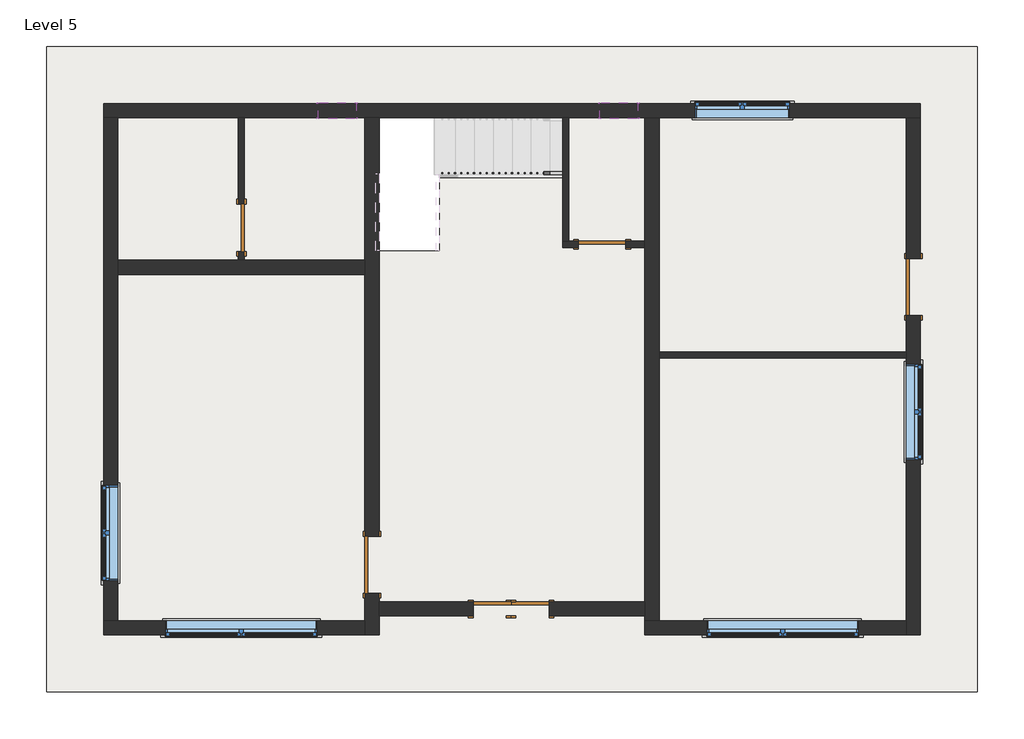
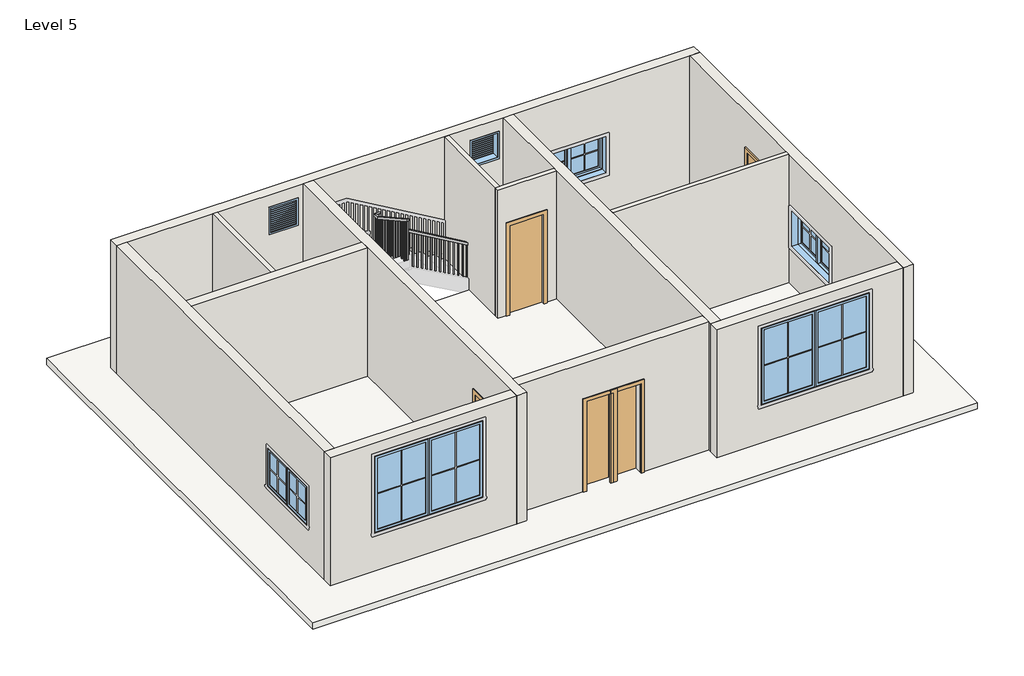
# One storey, part 1 of 2: 13 walls, 7 windows, 6 doors, 1 railing, 1 roof.
"""IFC4 building model written with IfcOpenShell, lengths in millimetres."""

from ifc_helpers import new_model, si_unit, frame, origin, place, context, project, spatial, polyline, outline, extrude, faceted_brep, transform, mapped, element, save
from components import single_flush_door_2_4a3212df, single_flush_door_2_0d3b4037, door_270f2424, door_aa9e95e7, single_flush_door_3_a90ba1ad, window_casement_double_c1d95f0f, window_casement_double_9ae172a2, window_f2d8fef0

model = new_model("IFC4")

# Units and contexts
model_context = context("Model", 3, world=origin())
ifc_project = project(units=[si_unit("LENGTHUNIT", "METRE", prefix="MILLI")], contexts=[model_context])

# Site, building, storey
site = spatial("IfcSite", under=ifc_project)
building = spatial("IfcBuilding", under=site)
storey = spatial("IfcBuildingStorey", under=building, Name="Level 5", Elevation=12649.2)

# Doors
placement = place(None, origin())
single_flush_door_2_shape = single_flush_door_2_4a3212df(model_context)
element("IfcDoor", 1, ObjectType="Single-Flush : DOOR 2'", at=placement, inside=storey, context=model_context, shape_type="MappedRepresentation", body=[
    mapped(single_flush_door_2_shape, transform((-1572.7415084, -2604.3618005, 12649.2), x_axis=(-1.0, 0.0, 0.0), y_axis=(0.0, -1.0, 0.0), z_axis=(0.0, 0.0, 1.0))),
])
single_flush_door_2_2_shape = single_flush_door_2_0d3b4037(model_context)
element("IfcDoor", 2, ObjectType="Single-Flush : DOOR 2'", at=placement, inside=storey, context=model_context, shape_type="MappedRepresentation", body=[
    mapped(single_flush_door_2_2_shape, transform((-963.1415084, -2604.3618005, 12649.2), x_axis=(1.0, 0.0, 0.0), y_axis=(0.0, 1.0, 0.0), z_axis=(0.0, 0.0, 1.0))),
])
door_shape = door_270f2424(model_context)
element("IfcDoor", 3, ObjectType="Single-Flush : DOOR 2'6\"", at=placement, inside=storey, context=model_context, shape_type="MappedRepresentation", body=[
    mapped(door_shape, transform((-5598.6415084, 3517.0381995, 12649.2), x_axis=(0.0, -1.0, 0.0), y_axis=(1.0, 0.0, 0.0), z_axis=(0.0, 0.0, 1.0))),
])
door_2_shape = door_aa9e95e7(model_context)
element("IfcDoor", 4, ObjectType="Single-Flush : DOOR 2'6\"", at=placement, inside=storey, context=model_context, shape_type="MappedRepresentation", body=[
    mapped(door_2_shape, transform((192.5584916, 3250.3381995, 12649.2), x_axis=(-1.0, 0.0, 0.0), y_axis=(0.0, -1.0, 0.0), z_axis=(0.0, 0.0, 1.0))),
])
single_flush_door_3_shape = single_flush_door_3_a90ba1ad(model_context)
element("IfcDoor", 5, ObjectType="Single-Flush : DOOR 3'", at=placement, inside=storey, context=model_context, shape_type="MappedRepresentation", body=[
    mapped(single_flush_door_3_shape, transform((-3503.1415084, -1893.1618005, 12649.2), x_axis=(0.0, -1.0, 0.0), y_axis=(1.0, 0.0, 0.0), z_axis=(0.0, 0.0, 1.0))),
])
element("IfcDoor", 6, ObjectType="Single-Flush : DOOR 3'", at=placement, inside=storey, context=model_context, shape_type="MappedRepresentation", body=[
    mapped(single_flush_door_3_shape, transform((5183.6584916, 2564.5381995, 12649.2), x_axis=(0.0, -1.0, 0.0), y_axis=(1.0, 0.0, 0.0), z_axis=(0.0, 0.0, 1.0))),
])

# Railing
element("IfcRailing", 7, ObjectType="Handrail - Rectangular", at=placement, inside=storey, context=model_context, shape_type="SolidModel", body=[
    faceted_brep([(-442.4415084, 4368.3146777, 13732.9333333), (-442.4415084, 4368.3146777, 13674.1219871), (-442.4415084, 4419.1146777, 13674.1219871), (-442.4415084, 4419.1146777, 13732.9333333), (-2398.2415084, 4368.3146777, 14873.8166667), (-2449.0415084, 4368.3146777, 14844.6386538), (-2449.0415084, 4419.1146777, 14844.6386538), (-2398.2415084, 4419.1146777, 14873.8166667), (-2398.2415084, 4368.3146777, 15129.9202697), (-2449.0415084, 4368.3146777, 15079.1202697), (-2449.0415084, 4419.1146777, 15079.1202697), (-2398.2415084, 4419.1146777, 15129.9202697), (-2474.4415084, 4368.3146777, 15129.9202697), (-2474.4415084, 4368.3146777, 15079.1202697), (-2525.2415084, 4419.1146777, 15079.1202697), (-2525.2415084, 4419.1146777, 15129.9202697), (-2474.4415084, 4292.1146777, 15129.9202697), (-2474.4415084, 4278.9546266, 15079.1202697), (-2525.2415084, 4278.9546266, 15079.1202697), (-2525.2415084, 4292.1146777, 15129.9202697), (-2474.4415084, 3148.7383287, 15764.9333333), (-2525.2415084, 3148.7383287, 15764.9333333), (-2525.2415084, 3148.7383287, 15706.82445), (-2474.4415084, 3148.7383287, 15706.82445)], [[[0, 1, 2, 3]], [[1, 0, 4, 5]], [[2, 1, 5, 6]], [[3, 2, 6, 7]], [[0, 3, 7, 4]], [[5, 4, 8, 9]], [[6, 5, 9, 10]], [[7, 6, 10, 11]], [[4, 7, 11, 8]], [[9, 8, 12, 13]], [[10, 9, 13, 14]], [[11, 10, 14, 15]], [[8, 11, 15, 12]], [[13, 12, 16, 17]], [[14, 13, 17, 18]], [[15, 14, 18, 19]], [[12, 15, 19, 16]], [[20, 21, 22, 23]], [[17, 16, 20, 23]], [[18, 17, 23, 22]], [[19, 18, 22, 21]], [[16, 19, 21, 20]]]),
    extrude(outline(polyline([(3184.0396777, 15687.3754052), (3184.0396777, 14681.2), (3164.9896777, 14681.2), (3164.9896777, 15697.9554726), (3184.0396777, 15687.3754052)])), frame((-2509.3665084, 0.0, 0.0), z_axis=(1.0, 0.0, 0.0), x_axis=(0.0, 1.0, 0.0)), (0.0, 0.0, 1.0), 19.05),
    extrude(outline(polyline([(3285.6396777, 15630.9483789), (3285.6396777, 14681.2), (3266.5896777, 14681.2), (3266.5896777, 15641.5284463), (3285.6396777, 15630.9483789)])), frame((-2509.3665084, 0.0, 0.0), z_axis=(1.0, 0.0, 0.0), x_axis=(0.0, 1.0, 0.0)), (0.0, 0.0, 1.0), 19.05),
    extrude(outline(polyline([(3387.2396777, 15574.5213526), (3387.2396777, 14681.2), (3368.1896777, 14681.2), (3368.1896777, 15585.1014201), (3387.2396777, 15574.5213526)])), frame((-2509.3665084, 0.0, 0.0), z_axis=(1.0, 0.0, 0.0), x_axis=(0.0, 1.0, 0.0)), (0.0, 0.0, 1.0), 19.05),
    extrude(outline(polyline([(3488.8396777, 15518.0420718), (3488.8396777, 14511.8666667), (3469.7896777, 14511.8666667), (3469.7896777, 15528.6221392), (3488.8396777, 15518.0420718)])), frame((-2509.3665084, 0.0, 0.0), z_axis=(1.0, 0.0, 0.0), x_axis=(0.0, 1.0, 0.0)), (0.0, 0.0, 1.0), 19.05),
    extrude(outline(polyline([(3590.4396777, 15461.6150456), (3590.4396777, 14511.8666667), (3571.3896777, 14511.8666667), (3571.3896777, 15472.195113), (3590.4396777, 15461.6150456)])), frame((-2509.3665084, 0.0, 0.0), z_axis=(1.0, 0.0, 0.0), x_axis=(0.0, 1.0, 0.0)), (0.0, 0.0, 1.0), 19.05),
    extrude(outline(polyline([(3692.0396777, 15405.1880193), (3692.0396777, 14511.8666667), (3672.9896777, 14511.8666667), (3672.9896777, 15415.7680867), (3692.0396777, 15405.1880193)])), frame((-2509.3665084, 0.0, 0.0), z_axis=(1.0, 0.0, 0.0), x_axis=(0.0, 1.0, 0.0)), (0.0, 0.0, 1.0), 19.05),
    extrude(outline(polyline([(3793.6396777, 15348.7087385), (3793.6396777, 14342.5333333), (3774.5896777, 14342.5333333), (3774.5896777, 15359.2888059), (3793.6396777, 15348.7087385)])), frame((-2509.3665084, 0.0, 0.0), z_axis=(1.0, 0.0, 0.0), x_axis=(0.0, 1.0, 0.0)), (0.0, 0.0, 1.0), 19.05),
    extrude(outline(polyline([(3895.2396777, 15292.2817122), (3895.2396777, 14342.5333333), (3876.1896777, 14342.5333333), (3876.1896777, 15302.8617797), (3895.2396777, 15292.2817122)])), frame((-2509.3665084, 0.0, 0.0), z_axis=(1.0, 0.0, 0.0), x_axis=(0.0, 1.0, 0.0)), (0.0, 0.0, 1.0), 19.05),
    extrude(outline(polyline([(3996.8396777, 15235.854686), (3996.8396777, 14342.5333333), (3977.7896777, 14342.5333333), (3977.7896777, 15246.4347534), (3996.8396777, 15235.854686)])), frame((-2509.3665084, 0.0, 0.0), z_axis=(1.0, 0.0, 0.0), x_axis=(0.0, 1.0, 0.0)), (0.0, 0.0, 1.0), 19.05),
    extrude(outline(polyline([(4098.4396777, 15179.3754052), (4098.4396777, 14173.2), (4079.3896777, 14173.2), (4079.3896777, 15189.9554726), (4098.4396777, 15179.3754052)])), frame((-2509.3665084, 0.0, 0.0), z_axis=(1.0, 0.0, 0.0), x_axis=(0.0, 1.0, 0.0)), (0.0, 0.0, 1.0), 19.05),
    extrude(outline(polyline([(4200.0396777, 15122.9483789), (4200.0396777, 14173.2), (4180.9896777, 14173.2), (4180.9896777, 15133.5284463), (4200.0396777, 15122.9483789)])), frame((-2509.3665084, 0.0, 0.0), z_axis=(1.0, 0.0, 0.0), x_axis=(0.0, 1.0, 0.0)), (0.0, 0.0, 1.0), 19.05),
    extrude(outline(polyline([(4301.6396777, 15066.5213526), (4301.6396777, 14173.2), (4282.5896777, 14173.2), (4282.5896777, 15077.1014201), (4301.6396777, 15066.5213526)])), frame((-2509.3665084, 0.0, 0.0), z_axis=(1.0, 0.0, 0.0), x_axis=(0.0, 1.0, 0.0)), (0.0, 0.0, 1.0), 19.05),
    extrude(outline(polyline([(-2464.9165084, 4384.1896777), (-2483.9665084, 4384.1896777), (-2483.9665084, 4403.2396777), (-2464.9165084, 4403.2396777), (-2464.9165084, 4384.1896777)])), frame((0.0, 0.0, 14003.8666667), z_axis=(0.0, 0.0, 1.0), x_axis=(1.0, 0.0, 0.0)), (0.0, 0.0, 1.0), 1075.253603),
    extrude(outline(polyline([(14805.7449038, -2382.3665084), (13834.5333333, -2382.3665084), (13834.5333333, -2363.3165084), (14794.6324038, -2363.3165084), (14805.7449038, -2382.3665084)])), frame((0.0, 4384.1896777, 0.0), z_axis=(0.0, 1.0, 0.0), x_axis=(0.0, 0.0, 1.0)), (0.0, 0.0, 1.0), 19.05),
    extrude(outline(polyline([(14746.4782371, -2280.7665084), (13834.5333333, -2280.7665084), (13834.5333333, -2261.7165084), (14735.3657371, -2261.7165084), (14746.4782371, -2280.7665084)])), frame((0.0, 4384.1896777, 0.0), z_axis=(0.0, 1.0, 0.0), x_axis=(0.0, 0.0, 1.0)), (0.0, 0.0, 1.0), 19.05),
    extrude(outline(polyline([(14687.2115704, -2179.1665084), (13834.5333333, -2179.1665084), (13834.5333333, -2160.1165084), (14676.0990704, -2160.1165084), (14687.2115704, -2179.1665084)])), frame((0.0, 4384.1896777, 0.0), z_axis=(0.0, 1.0, 0.0), x_axis=(0.0, 0.0, 1.0)), (0.0, 0.0, 1.0), 19.05),
    extrude(outline(polyline([(14627.9449038, -2077.5665084), (13665.2, -2077.5665084), (13665.2, -2058.5165084), (14616.8324038, -2058.5165084), (14627.9449038, -2077.5665084)])), frame((0.0, 4384.1896777, 0.0), z_axis=(0.0, 1.0, 0.0), x_axis=(0.0, 0.0, 1.0)), (0.0, 0.0, 1.0), 19.05),
    extrude(outline(polyline([(14568.6782371, -1975.9665084), (13665.2, -1975.9665084), (13665.2, -1956.9165084), (14557.5657371, -1956.9165084), (14568.6782371, -1975.9665084)])), frame((0.0, 4384.1896777, 0.0), z_axis=(0.0, 1.0, 0.0), x_axis=(0.0, 0.0, 1.0)), (0.0, 0.0, 1.0), 19.05),
    extrude(outline(polyline([(14509.4115704, -1874.3665084), (13665.2, -1874.3665084), (13665.2, -1855.3165084), (14498.2990704, -1855.3165084), (14509.4115704, -1874.3665084)])), frame((0.0, 4384.1896777, 0.0), z_axis=(0.0, 1.0, 0.0), x_axis=(0.0, 0.0, 1.0)), (0.0, 0.0, 1.0), 19.05),
    extrude(outline(polyline([(14450.1449038, -1772.7665084), (13495.8666667, -1772.7665084), (13495.8666667, -1753.7165084), (14439.0324038, -1753.7165084), (14450.1449038, -1772.7665084)])), frame((0.0, 4384.1896777, 0.0), z_axis=(0.0, 1.0, 0.0), x_axis=(0.0, 0.0, 1.0)), (0.0, 0.0, 1.0), 19.05),
    extrude(outline(polyline([(14390.8782371, -1671.1665084), (13495.8666667, -1671.1665084), (13495.8666667, -1652.1165084), (14379.7657371, -1652.1165084), (14390.8782371, -1671.1665084)])), frame((0.0, 4384.1896777, 0.0), z_axis=(0.0, 1.0, 0.0), x_axis=(0.0, 0.0, 1.0)), (0.0, 0.0, 1.0), 19.05),
    extrude(outline(polyline([(14331.6115704, -1569.5665084), (13495.8666667, -1569.5665084), (13495.8666667, -1550.5165084), (14320.4990704, -1550.5165084), (14331.6115704, -1569.5665084)])), frame((0.0, 4384.1896777, 0.0), z_axis=(0.0, 1.0, 0.0), x_axis=(0.0, 0.0, 1.0)), (0.0, 0.0, 1.0), 19.05),
    extrude(outline(polyline([(14272.3449038, -1467.9665084), (13326.5333333, -1467.9665084), (13326.5333333, -1448.9165084), (14261.2324038, -1448.9165084), (14272.3449038, -1467.9665084)])), frame((0.0, 4384.1896777, 0.0), z_axis=(0.0, 1.0, 0.0), x_axis=(0.0, 0.0, 1.0)), (0.0, 0.0, 1.0), 19.05),
    extrude(outline(polyline([(14213.0782371, -1366.3665084), (13326.5333333, -1366.3665084), (13326.5333333, -1347.3165084), (14201.9657371, -1347.3165084), (14213.0782371, -1366.3665084)])), frame((0.0, 4384.1896777, 0.0), z_axis=(0.0, 1.0, 0.0), x_axis=(0.0, 0.0, 1.0)), (0.0, 0.0, 1.0), 19.05),
    extrude(outline(polyline([(14153.8115704, -1264.7665084), (13326.5333333, -1264.7665084), (13326.5333333, -1245.7165084), (14142.6990704, -1245.7165084), (14153.8115704, -1264.7665084)])), frame((0.0, 4384.1896777, 0.0), z_axis=(0.0, 1.0, 0.0), x_axis=(0.0, 0.0, 1.0)), (0.0, 0.0, 1.0), 19.05),
    extrude(outline(polyline([(14094.5449038, -1163.1665084), (13157.2, -1163.1665084), (13157.2, -1144.1165084), (14083.4324038, -1144.1165084), (14094.5449038, -1163.1665084)])), frame((0.0, 4384.1896777, 0.0), z_axis=(0.0, 1.0, 0.0), x_axis=(0.0, 0.0, 1.0)), (0.0, 0.0, 1.0), 19.05),
    extrude(outline(polyline([(14035.2782371, -1061.5665084), (13157.2, -1061.5665084), (13157.2, -1042.5165084), (14024.1657371, -1042.5165084), (14035.2782371, -1061.5665084)])), frame((0.0, 4384.1896777, 0.0), z_axis=(0.0, 1.0, 0.0), x_axis=(0.0, 0.0, 1.0)), (0.0, 0.0, 1.0), 19.05),
    extrude(outline(polyline([(13976.0115704, -959.9665084), (13157.2, -959.9665084), (13157.2, -940.9165084), (13964.8990704, -940.9165084), (13976.0115704, -959.9665084)])), frame((0.0, 4384.1896777, 0.0), z_axis=(0.0, 1.0, 0.0), x_axis=(0.0, 0.0, 1.0)), (0.0, 0.0, 1.0), 19.05),
    extrude(outline(polyline([(13916.7449038, -858.3665084), (12987.8666667, -858.3665084), (12987.8666667, -839.3165084), (13905.6324038, -839.3165084), (13916.7449038, -858.3665084)])), frame((0.0, 4384.1896777, 0.0), z_axis=(0.0, 1.0, 0.0), x_axis=(0.0, 0.0, 1.0)), (0.0, 0.0, 1.0), 19.05),
    extrude(outline(polyline([(13857.4782371, -756.7665084), (12987.8666667, -756.7665084), (12987.8666667, -737.7165084), (13846.3657371, -737.7165084), (13857.4782371, -756.7665084)])), frame((0.0, 4384.1896777, 0.0), z_axis=(0.0, 1.0, 0.0), x_axis=(0.0, 0.0, 1.0)), (0.0, 0.0, 1.0), 19.05),
    extrude(outline(polyline([(13798.2115704, -655.1665084), (12987.8666667, -655.1665084), (12987.8666667, -636.1165084), (13787.0990704, -636.1165084), (13798.2115704, -655.1665084)])), frame((0.0, 4384.1896777, 0.0), z_axis=(0.0, 1.0, 0.0), x_axis=(0.0, 0.0, 1.0)), (0.0, 0.0, 1.0), 19.05),
    extrude(outline(polyline([(13738.9449038, -553.5665084), (12818.5333333, -553.5665084), (12818.5333333, -534.5165084), (13727.8324038, -534.5165084), (13738.9449038, -553.5665084)])), frame((0.0, 4384.1896777, 0.0), z_axis=(0.0, 1.0, 0.0), x_axis=(0.0, 0.0, 1.0)), (0.0, 0.0, 1.0), 19.05),
    extrude(outline(polyline([(-2490.3165084, 4384.1896777), (-2509.3665084, 4384.1896777), (-2509.3665084, 4403.2396777), (-2490.3165084, 4403.2396777), (-2490.3165084, 4384.1896777)])), frame((0.0, 0.0, 14003.8666667), z_axis=(0.0, 0.0, 1.0), x_axis=(1.0, 0.0, 0.0)), (0.0, 0.0, 1.0), 1075.253603),
    extrude(outline(polyline([(3167.7883287, 15696.2443826), (3167.7883287, 14681.2), (3148.7383287, 14681.2), (3148.7383287, 15706.82445), (3167.7883287, 15696.2443826)])), frame((-2509.3665084, 0.0, 0.0), z_axis=(1.0, 0.0, 0.0), x_axis=(0.0, 1.0, 0.0)), (0.0, 0.0, 1.0), 19.05),
    extrude(outline(polyline([(13685.2344871, -461.4915084), (12818.5333333, -461.4915084), (12818.5333333, -442.4415084), (13674.1219871, -442.4415084), (13685.2344871, -461.4915084)])), frame((0.0, 4384.1896777, 0.0), z_axis=(0.0, 1.0, 0.0), x_axis=(0.0, 0.0, 1.0)), (0.0, 0.0, 1.0), 19.05),
])

# Roof
element("IfcRoof", 8, ObjectType="ROOF 6\"", at=placement, inside=storey, context=model_context, shape_type="SweptSolid", body=[
    extrude(outline(polyline([(-8722.8415084, -3937.8618005), (-8722.8415084, 6425.3381995), (6212.3584916, 6425.3381995), (6212.3584916, -3937.8618005), (-8722.8415084, -3937.8618005)]), holes=[polyline([(-3439.6415084, 5333.1381995), (-3439.6415084, 3148.7383287), (-2423.6415084, 3148.7383287), (-2423.6415084, 4317.5146777), (-442.4415084, 4317.5146777), (-442.4415084, 5333.1381995), (-3439.6415084, 5333.1381995)])]), frame((0.0, 0.0, 12496.8), z_axis=(0.0, 0.0, 1.0), x_axis=(1.0, 0.0, 0.0)), (0.0, 0.0, 1.0), 152.4),
])

# Walls
element("IfcWall", 9, ObjectType="WALL 4\"", at=placement, inside=storey, context=model_context, shape_type="SweptSolid", body=[
    extrude(outline(polyline([(3136.0381995, 14782.8), (3136.0381995, 12649.2), (2996.3381995, 12649.2), (2996.3381995, 15697.2), (5282.3381995, 15697.2), (5282.3381995, 12649.2), (3898.0381995, 12649.2), (3898.0381995, 14782.8), (3136.0381995, 14782.8)])), frame((-5649.4415084, 0.0, 0.0), z_axis=(1.0, 0.0, 0.0), x_axis=(0.0, 1.0, 0.0)), (0.0, 0.0, 1.0), 101.6),
])
element("IfcWall", 10, ObjectType="WALL 4\"", at=placement, inside=storey, context=model_context, shape_type="Brep", body=[
    faceted_brep([(-188.4415084, 3301.1381995, 14782.8), (-188.4415084, 3301.1381995, 12649.2), (-340.8415084, 3301.1381995, 12649.2), (-442.4415084, 3301.1381995, 12649.2), (-442.4415084, 3301.1381995, 15697.2), (-340.8415084, 3301.1381995, 15697.2), (878.3584916, 3301.1381995, 15697.2), (878.3584916, 3301.1381995, 12649.2), (573.5584916, 3301.1381995, 12649.2), (573.5584916, 3301.1381995, 14782.8), (-442.4415084, 3199.5381995, 12649.2), (-188.4415084, 3199.5381995, 12649.2), (-188.4415084, 3199.5381995, 14782.8), (573.5584916, 3199.5381995, 14782.8), (573.5584916, 3199.5381995, 12649.2), (878.3584916, 3199.5381995, 12649.2), (878.3584916, 3199.5381995, 15697.2), (-442.4415084, 3199.5381995, 15697.2)], [[[0, 1, 2, 3, 4, 5, 6, 7, 8, 9]], [[10, 11, 12, 13, 14, 15, 16, 17]], [[8, 7, 15, 14]], [[3, 2, 1, 11, 10]], [[7, 6, 16, 15]], [[4, 3, 10, 17]], [[12, 11, 1, 0]], [[13, 12, 0, 9]], [[14, 13, 9, 8]], [[6, 5, 4, 17, 16]]]),
])
element("IfcWall", 11, ObjectType="WALL 4\"", at=placement, inside=storey, context=model_context, shape_type="Brep", body=[
    faceted_brep([(-340.8415084, 3301.1381995, 12649.2), (-340.8415084, 5282.3381995, 12649.2), (-340.8415084, 5282.3381995, 15697.2), (-340.8415084, 3301.1381995, 15697.2), (-442.4415084, 3301.1381995, 12649.2), (-442.4415084, 3301.1381995, 15697.2), (-442.4415084, 4317.5146777, 15697.2), (-442.4415084, 5282.3381995, 15697.2), (-442.4415084, 5282.3381995, 12649.2)], [[[0, 1, 2, 3]], [[4, 5, 6, 7, 8]], [[1, 0, 4, 8]], [[0, 3, 5, 4]], [[2, 1, 8, 7]], [[3, 2, 7, 6, 5]]]),
])
element("IfcWall", 12, ObjectType="WALL 4\"", at=placement, inside=storey, context=model_context, shape_type="SweptSolid", body=[
    extrude(outline(polyline([(1106.9584916, 1523.1381995), (5069.3584916, 1523.1381995), (5069.3584916, 1421.5381995), (1106.9584916, 1421.5381995), (1106.9584916, 1523.1381995)])), frame((0.0, 0.0, 12649.2), z_axis=(0.0, 0.0, 1.0), x_axis=(1.0, 0.0, 0.0)), (0.0, 0.0, 1.0), 3048.0),
])
element("IfcWall", 13, ObjectType="WALL 9\"", at=placement, inside=storey, context=model_context, shape_type="Brep", body=[
    faceted_brep([(-7808.4415084, 5282.3381995, 12649.2), (-7579.8415084, 5282.3381995, 12649.2), (-5649.4415084, 5282.3381995, 12649.2), (-5547.8415084, 5282.3381995, 12649.2), (-3617.4415084, 5282.3381995, 12649.2), (-3388.8415084, 5282.3381995, 12649.2), (-442.4415084, 5282.3381995, 12649.2), (-340.8415084, 5282.3381995, 12649.2), (878.3584916, 5282.3381995, 12649.2), (1106.9584916, 5282.3381995, 12649.2), (5069.3584916, 5282.3381995, 12649.2), (5297.9584916, 5282.3381995, 12649.2), (5297.9584916, 5282.3381995, 15697.2), (5069.3584916, 5282.3381995, 15697.2), (1106.9584916, 5282.3381995, 15697.2), (878.3584916, 5282.3381995, 15697.2), (-340.8415084, 5282.3381995, 15697.2), (-442.4415084, 5282.3381995, 15697.2), (-3388.8415084, 5282.3381995, 15697.2), (-3617.4415084, 5282.3381995, 15697.2), (-5547.8415084, 5282.3381995, 15697.2), (-5649.4415084, 5282.3381995, 15697.2), (-7579.8415084, 5282.3381995, 15697.2), (-7808.4415084, 5282.3381995, 15697.2), (3202.4584916, 5282.3381995, 14478.0), (3202.4584916, 5282.3381995, 13563.6), (1678.4584916, 5282.3381995, 13563.6), (1678.4584916, 5282.3381995, 14478.0), (154.4584916, 5282.3381995, 15392.4), (764.0584916, 5282.3381995, 15392.4), (764.0584916, 5282.3381995, 14782.8), (154.4584916, 5282.3381995, 14782.8), (-3757.1415084, 5282.3381995, 15392.4), (-3757.1415084, 5282.3381995, 14782.8), (-4366.7415084, 5282.3381995, 14782.8), (-4366.7415084, 5282.3381995, 15392.4), (-7808.4415084, 5510.9381995, 12649.2), (-7808.4415084, 5510.9381995, 15697.2), (5297.9584916, 5510.9381995, 15697.2), (5297.9584916, 5510.9381995, 12649.2), (3202.4584916, 5510.9381995, 14478.0), (1678.4584916, 5510.9381995, 14478.0), (1678.4584916, 5510.9381995, 13563.6), (3202.4584916, 5510.9381995, 13563.6), (154.4584916, 5510.9381995, 15392.4), (154.4584916, 5510.9381995, 14782.8), (764.0584916, 5510.9381995, 14782.8), (764.0584916, 5510.9381995, 15392.4), (-3757.1415084, 5510.9381995, 15392.4), (-4366.7415084, 5510.9381995, 15392.4), (-4366.7415084, 5510.9381995, 14782.8), (-3757.1415084, 5510.9381995, 14782.8)], [[[0, 1, 2, 3, 4, 5, 6, 7, 8, 9, 10, 11, 12, 13, 14, 15, 16, 17, 18, 19, 20, 21, 22, 23], [24, 25, 26, 27], [28, 29, 30, 31], [32, 33, 34, 35]], [[36, 37, 38, 39], [40, 41, 42, 43], [44, 45, 46, 47], [48, 49, 50, 51]], [[11, 10, 9, 8, 7, 6, 5, 4, 3, 2, 1, 0, 36, 39]], [[23, 22, 21, 20, 19, 18, 17, 16, 15, 14, 13, 12, 38, 37]], [[12, 11, 39, 38]], [[0, 23, 37, 36]], [[25, 24, 40, 43]], [[26, 25, 43, 42]], [[27, 26, 42, 41]], [[24, 27, 41, 40]], [[45, 44, 28, 31]], [[46, 45, 31, 30]], [[47, 46, 30, 29]], [[44, 47, 29, 28]], [[33, 32, 48, 51]], [[34, 33, 51, 50]], [[35, 34, 50, 49]], [[32, 35, 49, 48]]]),
])
element("IfcWall", 14, ObjectType="WALL 9\"", at=placement, inside=storey, context=model_context, shape_type="Brep", body=[
    faceted_brep([(5069.3584916, 2107.3381995, 14782.8), (5069.3584916, 2107.3381995, 12649.2), (5069.3584916, 1523.1381995, 12649.2), (5069.3584916, 1421.5381995, 12649.2), (5069.3584916, -2794.8618005, 12649.2), (5069.3584916, -3023.4618005, 12649.2), (5069.3584916, -3023.4618005, 15697.2), (5069.3584916, -2794.8618005, 15697.2), (5069.3584916, 1421.5381995, 15697.2), (5069.3584916, 1523.1381995, 15697.2), (5069.3584916, 5282.3381995, 15697.2), (5069.3584916, 5282.3381995, 12649.2), (5069.3584916, 3021.7381995, 12649.2), (5069.3584916, 3021.7381995, 14782.8), (5069.3584916, -204.0618005, 14478.0), (5069.3584916, -204.0618005, 13563.6), (5069.3584916, 1319.9381995, 13563.6), (5069.3584916, 1319.9381995, 14478.0), (5297.9584916, -3023.4618005, 12649.2), (5297.9584916, 2107.3381995, 12649.2), (5297.9584916, 2107.3381995, 14782.8), (5297.9584916, 3021.7381995, 14782.8), (5297.9584916, 3021.7381995, 12649.2), (5297.9584916, 5282.3381995, 12649.2), (5297.9584916, 5282.3381995, 15697.2), (5297.9584916, -3023.4618005, 15697.2), (5297.9584916, -204.0618005, 14478.0), (5297.9584916, 1319.9381995, 14478.0), (5297.9584916, 1319.9381995, 13563.6), (5297.9584916, -204.0618005, 13563.6)], [[[0, 1, 2, 3, 4, 5, 6, 7, 8, 9, 10, 11, 12, 13], [14, 15, 16, 17]], [[18, 19, 20, 21, 22, 23, 24, 25], [26, 27, 28, 29]], [[12, 11, 23, 22]], [[5, 4, 3, 2, 1, 19, 18]], [[11, 10, 24, 23]], [[6, 5, 18, 25]], [[15, 14, 26, 29]], [[16, 15, 29, 28]], [[17, 16, 28, 27]], [[14, 17, 27, 26]], [[20, 19, 1, 0]], [[21, 20, 0, 13]], [[22, 21, 13, 12]], [[10, 9, 8, 7, 6, 25, 24]]]),
])
element("IfcWall", 15, ObjectType="WALL 9\"", at=placement, inside=storey, context=model_context, shape_type="Brep", body=[
    faceted_brep([(5069.3584916, -2794.8618005, 12649.2), (1106.9584916, -2794.8618005, 12649.2), (878.3584916, -2794.8618005, 12649.2), (878.3584916, -2794.8618005, 15697.2), (1106.9584916, -2794.8618005, 15697.2), (5069.3584916, -2794.8618005, 15697.2), (1868.9584916, -2794.8618005, 15392.4), (1868.9584916, -2794.8618005, 13563.6), (4307.3584916, -2794.8618005, 13563.6), (4307.3584916, -2794.8618005, 15392.4), (5069.3584916, -3023.4618005, 12649.2), (5069.3584916, -3023.4618005, 15697.2), (878.3584916, -3023.4618005, 15697.2), (878.3584916, -3023.4618005, 12649.2), (1868.9584916, -3023.4618005, 15392.4), (4307.3584916, -3023.4618005, 15392.4), (4307.3584916, -3023.4618005, 13563.6), (1868.9584916, -3023.4618005, 13563.6)], [[[0, 1, 2, 3, 4, 5], [6, 7, 8, 9]], [[10, 11, 12, 13], [14, 15, 16, 17]], [[2, 1, 0, 10, 13]], [[0, 5, 11, 10]], [[3, 2, 13, 12]], [[7, 6, 14, 17]], [[8, 7, 17, 16]], [[9, 8, 16, 15]], [[6, 9, 15, 14]], [[5, 4, 3, 12, 11]]]),
])
element("IfcWall", 16, ObjectType="WALL 9\"", at=placement, inside=storey, context=model_context, shape_type="Brep", body=[
    faceted_brep([(1106.9584916, -2794.8618005, 12649.2), (1106.9584916, 1421.5381995, 12649.2), (1106.9584916, 1523.1381995, 12649.2), (1106.9584916, 5282.3381995, 12649.2), (1106.9584916, 5282.3381995, 15697.2), (1106.9584916, 1523.1381995, 15697.2), (1106.9584916, 1421.5381995, 15697.2), (1106.9584916, -2794.8618005, 15697.2), (878.3584916, -2794.8618005, 12649.2), (878.3584916, -2794.8618005, 15697.2), (878.3584916, -2718.6618005, 15697.2), (878.3584916, -2490.0618005, 15697.2), (878.3584916, 3199.5381995, 15697.2), (878.3584916, 3301.1381995, 15697.2), (878.3584916, 5282.3381995, 15697.2), (878.3584916, 5282.3381995, 12649.2), (878.3584916, 3301.1381995, 12649.2), (878.3584916, 3199.5381995, 12649.2), (878.3584916, -2490.0618005, 12649.2), (878.3584916, -2718.6618005, 12649.2)], [[[0, 1, 2, 3, 4, 5, 6, 7]], [[8, 9, 10, 11, 12, 13, 14, 15, 16, 17, 18, 19]], [[3, 2, 1, 0, 8, 19, 18, 17, 16, 15]], [[0, 7, 9, 8]], [[4, 3, 15, 14]], [[7, 6, 5, 4, 14, 13, 12, 11, 10, 9]]]),
])
element("IfcWall", 17, ObjectType="WALL 9\"", at=placement, inside=storey, context=model_context, shape_type="SweptSolid", body=[
    extrude(outline(polyline([(12649.2, 878.3584916), (15697.2, 878.3584916), (15697.2, -3388.8415084), (12649.2, -3388.8415084), (12649.2, -1877.5415084), (14782.8, -1877.5415084), (14782.8, -658.3415084), (12649.2, -658.3415084), (12649.2, 878.3584916)])), frame((0.0, -2718.6618005, 0.0), z_axis=(0.0, 1.0, 0.0), x_axis=(0.0, 0.0, 1.0)), (0.0, 0.0, 1.0), 228.6),
])
element("IfcWall", 18, ObjectType="WALL 9\"", at=placement, inside=storey, context=model_context, shape_type="Brep", body=[
    faceted_brep([(-3388.8415084, -3023.4618005, 12649.2), (-3388.8415084, -2718.6618005, 12649.2), (-3388.8415084, -2490.0618005, 12649.2), (-3388.8415084, -2350.3618005, 12649.2), (-3388.8415084, -2350.3618005, 14782.8), (-3388.8415084, -1435.9618005, 14782.8), (-3388.8415084, -1435.9618005, 12649.2), (-3388.8415084, 5282.3381995, 12649.2), (-3388.8415084, 5282.3381995, 15697.2), (-3388.8415084, -2490.0618005, 15697.2), (-3388.8415084, -2718.6618005, 15697.2), (-3388.8415084, -3023.4618005, 15697.2), (-3617.4415084, -2350.3618005, 14782.8), (-3617.4415084, -2350.3618005, 12649.2), (-3617.4415084, -2794.8618005, 12649.2), (-3617.4415084, -3023.4618005, 12649.2), (-3617.4415084, -3023.4618005, 15697.2), (-3617.4415084, -2794.8618005, 15697.2), (-3617.4415084, 2767.7381995, 15697.2), (-3617.4415084, 2996.3381995, 15697.2), (-3617.4415084, 5282.3381995, 15697.2), (-3617.4415084, 5282.3381995, 12649.2), (-3617.4415084, 2996.3381995, 12649.2), (-3617.4415084, 2767.7381995, 12649.2), (-3617.4415084, -1435.9618005, 12649.2), (-3617.4415084, -1435.9618005, 14782.8)], [[[0, 1, 2, 3, 4, 5, 6, 7, 8, 9, 10, 11]], [[12, 13, 14, 15, 16, 17, 18, 19, 20, 21, 22, 23, 24, 25]], [[15, 14, 13, 3, 2, 1, 0]], [[24, 23, 22, 21, 7, 6]], [[11, 10, 9, 8, 20, 19, 18, 17, 16]], [[8, 7, 21, 20]], [[0, 11, 16, 15]], [[4, 3, 13, 12]], [[5, 4, 12, 25]], [[6, 5, 25, 24]]]),
])
element("IfcWall", 19, ObjectType="WALL 9\"", at=placement, inside=storey, context=model_context, shape_type="Brep", body=[
    faceted_brep([(-3617.4415084, -2794.8618005, 12649.2), (-7579.8415084, -2794.8618005, 12649.2), (-7808.4415084, -2794.8618005, 12649.2), (-7808.4415084, -2794.8618005, 15697.2), (-7579.8415084, -2794.8618005, 15697.2), (-3617.4415084, -2794.8618005, 15697.2), (-6817.8415084, -2794.8618005, 15392.4), (-6817.8415084, -2794.8618005, 13563.6), (-4379.4415084, -2794.8618005, 13563.6), (-4379.4415084, -2794.8618005, 15392.4), (-3617.4415084, -3023.4618005, 12649.2), (-3617.4415084, -3023.4618005, 15697.2), (-7808.4415084, -3023.4618005, 15697.2), (-7808.4415084, -3023.4618005, 12649.2), (-6817.8415084, -3023.4618005, 15392.4), (-4379.4415084, -3023.4618005, 15392.4), (-4379.4415084, -3023.4618005, 13563.6), (-6817.8415084, -3023.4618005, 13563.6)], [[[0, 1, 2, 3, 4, 5], [6, 7, 8, 9]], [[10, 11, 12, 13], [14, 15, 16, 17]], [[2, 1, 0, 10, 13]], [[0, 5, 11, 10]], [[3, 2, 13, 12]], [[7, 6, 14, 17]], [[8, 7, 17, 16]], [[9, 8, 16, 15]], [[6, 9, 15, 14]], [[5, 4, 3, 12, 11]]]),
])
element("IfcWall", 20, ObjectType="WALL 9\"", at=placement, inside=storey, context=model_context, shape_type="Brep", body=[
    faceted_brep([(-7579.8415084, -2794.8618005, 12649.2), (-7579.8415084, 2767.7381995, 12649.2), (-7579.8415084, 2996.3381995, 12649.2), (-7579.8415084, 5282.3381995, 12649.2), (-7579.8415084, 5282.3381995, 15697.2), (-7579.8415084, 2996.3381995, 15697.2), (-7579.8415084, 2767.7381995, 15697.2), (-7579.8415084, -2794.8618005, 15697.2), (-7579.8415084, -623.1618005, 14478.0), (-7579.8415084, -623.1618005, 13563.6), (-7579.8415084, -2147.1618005, 13563.6), (-7579.8415084, -2147.1618005, 14478.0), (-7808.4415084, -2794.8618005, 12649.2), (-7808.4415084, -2794.8618005, 15697.2), (-7808.4415084, 5282.3381995, 15697.2), (-7808.4415084, 5282.3381995, 12649.2), (-7808.4415084, -623.1618005, 14478.0), (-7808.4415084, -2147.1618005, 14478.0), (-7808.4415084, -2147.1618005, 13563.6), (-7808.4415084, -623.1618005, 13563.6)], [[[0, 1, 2, 3, 4, 5, 6, 7], [8, 9, 10, 11]], [[12, 13, 14, 15], [16, 17, 18, 19]], [[3, 2, 1, 0, 12, 15]], [[0, 7, 13, 12]], [[4, 3, 15, 14]], [[9, 8, 16, 19]], [[10, 9, 19, 18]], [[11, 10, 18, 17]], [[8, 11, 17, 16]], [[7, 6, 5, 4, 14, 13]]]),
])
element("IfcWall", 21, ObjectType="WALL 9\"", at=placement, inside=storey, context=model_context, shape_type="Brep", body=[
    faceted_brep([(-7579.8415084, 2767.7381995, 12649.2), (-3617.4415084, 2767.7381995, 12649.2), (-3617.4415084, 2767.7381995, 15697.2), (-7579.8415084, 2767.7381995, 15697.2), (-7579.8415084, 2996.3381995, 12649.2), (-7579.8415084, 2996.3381995, 15697.2), (-5649.4415084, 2996.3381995, 15697.2), (-5547.8415084, 2996.3381995, 15697.2), (-3617.4415084, 2996.3381995, 15697.2), (-3617.4415084, 2996.3381995, 12649.2), (-5547.8415084, 2996.3381995, 12649.2), (-5649.4415084, 2996.3381995, 12649.2)], [[[0, 1, 2, 3]], [[4, 5, 6, 7, 8, 9, 10, 11]], [[1, 0, 4, 11, 10, 9]], [[2, 1, 9, 8]], [[0, 3, 5, 4]], [[3, 2, 8, 7, 6, 5]]]),
])

# Windows
window_casement_double_shape = window_casement_double_c1d95f0f(model_context)
element("IfcWindow", 22, ObjectType="Window-Casement-Double", at=placement, inside=storey, context=model_context, shape_type="MappedRepresentation", body=[
    mapped(window_casement_double_shape, transform((-7694.1415084, -1385.1618005, 12649.2), x_axis=(0.0, 1.0, 0.0), y_axis=(-1.0, 0.0, 0.0), z_axis=(0.0, 0.0, 1.0))),
])
element("IfcWindow", 23, ObjectType="Window-Casement-Double", at=placement, inside=storey, context=model_context, shape_type="MappedRepresentation", body=[
    mapped(window_casement_double_shape, transform((5183.6584916, 557.9381995, 12649.2), x_axis=(0.0, -1.0, 0.0), y_axis=(1.0, 0.0, 0.0), z_axis=(0.0, 0.0, 1.0))),
])
element("IfcWindow", 24, ObjectType="Window-Casement-Double", at=placement, inside=storey, context=model_context, shape_type="MappedRepresentation", body=[
    mapped(window_casement_double_shape, transform((2440.4584916, 5396.6381995, 12649.2), x_axis=(1.0, 0.0, 0.0), y_axis=(0.0, 1.0, 0.0), z_axis=(0.0, 0.0, 1.0))),
])
window_casement_double_2_shape = window_casement_double_9ae172a2(model_context)
element("IfcWindow", 25, ObjectType="Window-Casement-Double", at=placement, inside=storey, context=model_context, shape_type="MappedRepresentation", body=[
    mapped(window_casement_double_2_shape, transform((-5598.6415084, -2909.1618005, 12649.2), x_axis=(-1.0, 0.0, 0.0), y_axis=(0.0, -1.0, 0.0), z_axis=(0.0, 0.0, 1.0))),
])
element("IfcWindow", 26, ObjectType="Window-Casement-Double", at=placement, inside=storey, context=model_context, shape_type="MappedRepresentation", body=[
    mapped(window_casement_double_2_shape, transform((3088.1584916, -2909.1618005, 12649.2), x_axis=(-1.0, 0.0, 0.0), y_axis=(0.0, -1.0, 0.0), z_axis=(0.0, 0.0, 1.0))),
])
window_shape = window_f2d8fef0(model_context)
element("IfcWindow", 27, ObjectType="Window-Louvers : 24\" x 24\"", at=placement, inside=storey, context=model_context, shape_type="MappedRepresentation", body=[
    mapped(window_shape, transform((459.2584916, 5402.9881995, 13868.4), x_axis=(1.0, 0.0, 0.0), y_axis=(0.0, 1.0, 0.0), z_axis=(0.0, 0.0, 1.0))),
])
element("IfcWindow", 28, ObjectType="Window-Louvers : 24\" x 24\"", at=placement, inside=storey, context=model_context, shape_type="MappedRepresentation", body=[
    mapped(window_shape, transform((-4061.9415084, 5390.2881995, 13868.4), x_axis=(-1.0, 0.0, 0.0), y_axis=(0.0, -1.0, 0.0), z_axis=(0.0, 0.0, 1.0))),
])

save(model, "model.ifc")

# Revit data of these elements
# Type "Single-Flush : DOOR 2'"
#   Type Mark = "10"
#   Construction Type Id = "MDOOR"
#   Assembly Code = "C1020"
#   Analytic Construction = "Metal"
#   Thickness = 0' - 2"
#   Heat Transfer Coefficient (U) = 0.651978 BTU/(h·ft²·°F)
#   Height = 7' - 0"
#   Trim Projection Ext = 0' - 1"
#   Trim Projection Int = 0' - 1"
#   Trim Width = 0' - 3"
#   Width = 2' - 0"
#   Define Thermal Properties by = 1
#   Door Material = Door - Panel
#   Frame Material = Door - Frame
#   Visual Light Transmittance = 0
#   Solar Heat Gain Coefficient = 0
#   Function = (empty or 0)
#   Wall Closure = (empty or 0)
# Type "Single-Flush : DOOR 2'6\""
#   Type Mark = "9"
#   Construction Type Id = "MDOOR"
#   Assembly Code = "C1020"
#   Analytic Construction = "Metal"
#   Thickness = 0' - 2"
#   Heat Transfer Coefficient (U) = 0.651978 BTU/(h·ft²·°F)
#   Height = 7' - 0"
#   Trim Projection Ext = 0' - 1"
#   Trim Projection Int = 0' - 1"
#   Trim Width = 0' - 3"
#   Width = 2' - 6"
#   Define Thermal Properties by = 1
#   Door Material = Door - Panel
#   Frame Material = Door - Frame
#   Visual Light Transmittance = 0
#   Solar Heat Gain Coefficient = 0
#   Function = (empty or 0)
#   Wall Closure = (empty or 0)
# Type "Single-Flush : DOOR 3'"
#   Type Mark = "8"
#   Construction Type Id = "MDOOR"
#   Assembly Code = "C1020"
#   Analytic Construction = "Metal"
#   Thickness = 0' - 2"
#   Heat Transfer Coefficient (U) = 0.651978 BTU/(h·ft²·°F)
#   Height = 7' - 0"
#   Trim Projection Ext = 0' - 1"
#   Trim Projection Int = 0' - 1"
#   Trim Width = 0' - 3"
#   Width = 3' - 0"
#   Define Thermal Properties by = 1
#   Door Material = Door - Panel
#   Frame Material = Door - Frame
#   Visual Light Transmittance = 0
#   Solar Heat Gain Coefficient = 0
#   Function = (empty or 0)
#   Wall Closure = (empty or 0)
# Type "Handrail - Rectangular"
#   Assembly Code = "C2010400"
#   built-in parameter 1008612 = 0.0416667 (stored number, unit not read)
#   built-in parameter 1008611 = 0.0416667 (stored number, unit not read)
#   built-in parameter 1008609 = 0.333333 (stored number, unit not read)
#   built-in parameter 1008604 = 0.166667 (stored number, unit not read)
#   built-in parameter 1008603 = 0.166667 (stored number, unit not read)
#   Railing Height = 3' - 0"
#   built-in parameter 1008630 = 2
#   built-in parameter 1008610 = 2
#   built-in parameter 1008618 = Baluster - Square : 3/4"
# Type "ROOF 6\""
#   Assembly Code = "B1020"
#   Layers, outside or top first: 0' - 6" no material (function 1)
# Type "WALL 4\""
#   Assembly Code = "B2010"
#   Layers, outside or top first: 0' - 4" no material (function 1)
# Type "WALL 9\""
#   Assembly Code = "B2010"
#   Layers, outside or top first: 0' - 9" no material (function 1)
# Type "Window-Casement-Double"
#   Type Mark = "18"
#   Fire Rating = "0.5h"
#   Assembly Code = "B2020100"
#   Analytic Construction = "Double glazing - domestic"
#   Frame Extension [instance default] = 0' - 0 1/4"
#   Window Inset [instance default] = 0' - 0"
#   Wall Thickness [instance default] = 0' - 6"
#   Interior Wall Closure [instance default] = 0' - 2 1/4"
#   Half Width = 2' - 6"
#   Visual Light Transmittance = 0.81
#   Thermal Resistance (R) = 1.8146 (h·ft²·°F)/BTU
#   Solar Heat Gain Coefficient = 0.76
#   Rough Width = 5' - 0 1/2"
#   Rough Height = 3' - 0 1/2"
#   Height = 3' - 0"
#   Heat Transfer Coefficient (U) = 0.5511 BTU/(h·ft²·°F)
#   Exterior Wall Closure [instance default] = 0' - 1 1/4"
#   Extension Jamb [instance default] = 0' - 2 1/4"
#   Default Sill Height = 3' - 0"
#   Width = 5' - 0"
#   Muntin Visibility = yes
#   Interior Trim Visibility [instance default] = yes
#   Exterior Trim Visibility [instance default] = yes
#   Extension Jamb Visibility [instance default] = yes
#   Interior Trim Material = Wood - Stained
#   Muntin Pattern = Muntin Pattern_2x2 : Muntin Pattern_2x2
#   Interior Trim = Trim-Window-Interior-Flat : Picture Frame
#   Interior Frame Material = Wood - Stained
#   Glass Panel Material = Glass
#   Exterior Trim Material = Clad - White
#   Exterior Trim = Trim-Window-Exterior-Flat : with Sill
#   Exterior Frame Material = Clad - White
#   Wall Closure = (empty or 0)
# Type "Window-Casement-Double"
#   Type Mark = "19"
#   Fire Rating = "0.5h"
#   Assembly Code = "B2020100"
#   Analytic Construction = "Double glazing - domestic"
#   Frame Extension [instance default] = 0' - 0 1/4"
#   Window Inset [instance default] = 0' - 0"
#   Wall Thickness [instance default] = 0' - 6"
#   Interior Wall Closure [instance default] = 0' - 2 1/4"
#   Half Width = 4' - 0"
#   Visual Light Transmittance = 0.81
#   Thermal Resistance (R) = 1.8146 (h·ft²·°F)/BTU
#   Solar Heat Gain Coefficient = 0.76
#   Rough Width = 8' - 0 1/2"
#   Rough Height = 6' - 0 1/2"
#   Height = 6' - 0"
#   Heat Transfer Coefficient (U) = 0.5511 BTU/(h·ft²·°F)
#   Exterior Wall Closure [instance default] = 0' - 1 1/4"
#   Extension Jamb [instance default] = 0' - 2 1/4"
#   Default Sill Height = 3' - 0"
#   Width = 8' - 0"
#   Muntin Visibility = yes
#   Interior Trim Visibility [instance default] = yes
#   Exterior Trim Visibility [instance default] = yes
#   Extension Jamb Visibility [instance default] = yes
#   Interior Trim Material = Wood - Stained
#   Muntin Pattern = Muntin Pattern_2x2 : Muntin Pattern_2x2
#   Interior Trim = Trim-Window-Interior-Flat : Picture Frame
#   Interior Frame Material = Wood - Stained
#   Glass Panel Material = Glass
#   Exterior Trim Material = Clad - White
#   Exterior Trim = Trim-Window-Exterior-Flat : with Sill
#   Exterior Frame Material = Clad - White
#   Wall Closure = (empty or 0)
# Type "Window-Louvers : 24\" x 24\""
#   Type Mark = "20"
#   Construction Type Id = "GSP4R"
#   Assembly Code = "B20"
#   Analytic Construction = "1/8 in Pilkington single glazing"
#   Visual Light Transmittance = 0.9
#   Thermal Resistance (R) = 1.53941 (h·ft²·°F)/BTU
#   Solar Heat Gain Coefficient = 0.78
#   Max Height = 1' - 11.74264"
#   Height = 2' - 0"
#   Heat Transfer Coefficient (U) = 0.6496 BTU/(h·ft²·°F)
#   Blade Width [instance default] = 1' - 10 1/2"
#   Blade Vertical Thickness = 0' - 0.35355"
#   Blade Thickness = 0' - 0 1/4"
#   Blade Spacing = 0' - 1 1/2"
#   Blade Height = 0' - 1.85355"
#   Blade Depth = 0' - 3"
#   Blade Angle = 45.00°
#   Default Sill Height = 3' - 0"
#   Trim Projection_Exterior = 0' - 0 1/2"
#   Trim Projection_Interior = 0' - 0 1/2"
#   Trim Width_Exterior = 0' - 1 1/2"
#   Trim Width_Interior = 0' - 1 1/2"
#   Width = 2' - 0"
#   Max Blade Count = 12
#   Define Thermal Properties by = 1
#   Blade Count = 12
#   Frame Material = Birch
#   Louver Material = Birch
#   Trim Exterior Material = Birch
#   Trim Interior Material = Birch
#   Wall Closure = (empty or 0)
# Elements 1, 2 (IfcDoor, "Single-Flush : DOOR 2'")
#   Phase Created = New Construction
#   Materials on its faces: "Door - Frame", "Door - Panel"
# Elements 3, 4 (IfcDoor, "Single-Flush : DOOR 2'6\"")
#   Phase Created = New Construction
#   Materials on its faces: "Door - Frame", "Door - Panel"
# Elements 5, 6 (IfcDoor, "Single-Flush : DOOR 3'")
#   Phase Created = New Construction
#   Materials on its faces: "Door - Frame", "Door - Panel"
# Element 7 (IfcRailing, "Handrail - Rectangular")
#   Phase Created = New Construction
# Element 8 (IfcRoof, "ROOF 6\"")
#   built-in parameter 1001705 = 41.5 (stored number, unit not read)
#   built-in parameter 1001701 = -0.5 (stored number, unit not read)
#   built-in parameter 1001710 = 33615
#   Phase Created = New Construction
#   Materials on its faces: "Door - Frame", "Default Roof", "Wood - Stained"
# Elements 9, 12 (IfcWall, "WALL 4\"")
#   Top Offset = 0' - 0"
#   Base Offset = 0' - 0"
#   Unconnected Height = 10' - 0"
#   wall height = 10' - 0"
#   Phase Created = New Construction
#   Base Constraint = Level 5
#   Materials on its faces: "Default Wall"
# Elements 10, 11 (IfcWall, "WALL 4\"")
#   Top Offset = 0' - 0"
#   Base Offset = 0' - 0"
#   Unconnected Height = 10' - 0"
#   wall height = 10' - 0"
#   Phase Created = New Construction
#   Base Constraint = Level 5
#   Materials on its faces: "Default Wall", "Door - Frame"
# Element 13 (IfcWall, "WALL 9\"")
#   Top Offset = 0' - 0"
#   Base Offset = 0' - 0"
#   Unconnected Height = 10' - 0"
#   wall height = 10' - 0"
#   Phase Created = New Construction
#   Base Constraint = Level 5
#   Materials on its faces: "Default Wall", "Parking Stripe", "Door - Frame"
# Elements 14, 15, 16, 17, 19, 20 (IfcWall, "WALL 9\"")
#   Top Offset = 0' - 0"
#   Base Offset = 0' - 0"
#   Unconnected Height = 10' - 0"
#   wall height = 10' - 0"
#   Phase Created = New Construction
#   Base Constraint = Level 5
#   Materials on its faces: "Default Wall", "Parking Stripe"
# Element 18 (IfcWall, "WALL 9\"")
#   Top Offset = 0' - 0"
#   Base Offset = 0' - 0"
#   Unconnected Height = 10' - 0"
#   wall height = 10' - 0"
#   Phase Created = New Construction
#   Base Constraint = Level 5
#   Materials on its faces: "Default Wall", "Door - Frame", "Parking Stripe"
# Element 21 (IfcWall, "WALL 9\"")
#   Top Offset = 0' - 0"
#   Base Offset = 0' - 0"
#   Unconnected Height = 10' - 0"
#   wall height = 10' - 0"
#   Phase Created = New Construction
#   Base Constraint = Level 5
#   Materials on its faces: "Default Wall"
# Element 22 (IfcWindow, "Window-Casement-Double")
#   Mark = "29"
#   Window Inset = 0' - 0"
#   Interior Wall Closure = 0' - 2 1/4"
#   Frame Extension = 0' - 0 1/4"
#   Exterior Wall Closure = 0' - 1 1/4"
#   Interior Trim Visibility = yes
#   Exterior Trim Visibility = yes
#   Phase Created = New Construction
#   Materials on its faces: "Wood - Stained", "Glass", "Clad - White"
# Element 23 (IfcWindow, "Window-Casement-Double")
#   Mark = "30"
#   Window Inset = 0' - 0"
#   Interior Wall Closure = 0' - 2 1/4"
#   Frame Extension = 0' - 0 1/4"
#   Exterior Wall Closure = 0' - 1 1/4"
#   Interior Trim Visibility = yes
#   Exterior Trim Visibility = yes
#   Phase Created = New Construction
#   Materials on its faces: "Wood - Stained", "Glass", "Clad - White"
# Element 24 (IfcWindow, "Window-Casement-Double")
#   Mark = "31"
#   Window Inset = 0' - 0"
#   Interior Wall Closure = 0' - 2 1/4"
#   Frame Extension = 0' - 0 1/4"
#   Exterior Wall Closure = 0' - 1 1/4"
#   Interior Trim Visibility = yes
#   Exterior Trim Visibility = yes
#   Phase Created = New Construction
#   Materials on its faces: "Wood - Stained", "Glass", "Clad - White"
# Element 25 (IfcWindow, "Window-Casement-Double")
#   Mark = "32"
#   Window Inset = 0' - 0"
#   Interior Wall Closure = 0' - 2 1/4"
#   Frame Extension = 0' - 0 1/4"
#   Exterior Wall Closure = 0' - 1 1/4"
#   Interior Trim Visibility = yes
#   Exterior Trim Visibility = yes
#   Phase Created = New Construction
#   Materials on its faces: "Wood - Stained", "Glass", "Clad - White"
# Element 26 (IfcWindow, "Window-Casement-Double")
#   Mark = "33"
#   Window Inset = 0' - 0"
#   Interior Wall Closure = 0' - 2 1/4"
#   Frame Extension = 0' - 0 1/4"
#   Exterior Wall Closure = 0' - 1 1/4"
#   Interior Trim Visibility = yes
#   Exterior Trim Visibility = yes
#   Phase Created = New Construction
#   Materials on its faces: "Wood - Stained", "Glass", "Clad - White"
# Element 27 (IfcWindow, "Window-Louvers : 24\" x 24\"")
#   Mark = "34"
#   Blade Width = 1' - 10 1/2"
#   Phase Created = New Construction
#   Materials on its faces: "Birch"
# Element 28 (IfcWindow, "Window-Louvers : 24\" x 24\"")
#   Mark = "35"
#   Blade Width = 1' - 10 1/2"
#   Phase Created = New Construction
#   Materials on its faces: "Birch"
# Materials
#   "Door - Panel": class "Wood", colour RGB 210 159 95, transparency 0, Cost = 0
#   "Door - Frame": colour RGB 118 70 51, transparency 0, Cost = 0
#   "Wood - Stained": class "Wood", colour RGB 224 178 126, transparency 0, Cost = 0
#   "Glass": class "Glass", colour RGB 0 128 192, transparency 0.75, Description = "Soda Lime Glass", Cost = 0
#   "Clad - White": class "Wood", colour RGB 242 242 238, transparency 0, Cost = 0
#   "Birch": class "Wood", colour RGB 224 178 126, transparency 0, Description = "Betula Alleghaniensis", Cost = 0
#   "Default Roof": colour RGB 88 101 114, transparency 0, Cost = 0
#   "Default Wall": colour RGB 128 128 128, transparency 0, Cost = 0
#   "Parking Stripe": class "Paint", colour RGB 250 250 91, transparency 0, Cost = 0
